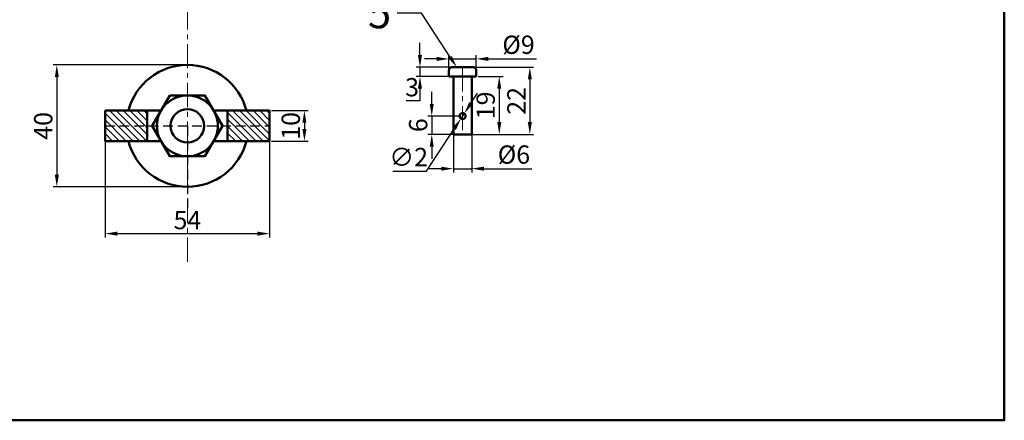
# Model space of a CAD drawing. Units: millimetres. Extents: x -25 to 763, y -62 to 306.
# Tile 5 of 7: x 440 to 763, y -62 to 69. Entities that reach past the tile are written whole.
import ezdxf
from ezdxf import colors
from ezdxf.entities.mleader import LeaderData, LeaderLine
from ezdxf.math import Vec2, Vec3

# ---------------------------------------------------------------- set-up
doc = ezdxf.new("R2010")
doc.units = ezdxf.units.MM
doc.header["$LTSCALE"] = 0.5
doc.linetypes.add('CENTER', pattern=[50.8, 31.75, -6.35, 6.35, -6.35])
doc.linetypes.add('DASHED', pattern=[19.05, 12.7, -6.35])
for name, color, linetype, lineweight in [('M-CNTR', 1, 'CENTER', 18), ('M-DIMS', 2, 'Continuous', 25), ('M-HATC', 8, 'Continuous', 18), ('M-HIDN', 4, 'DASHED', 25), ('M-OUTL', 7, 'Continuous', 50), ('M-TEXT', 3, 'Continuous', 25), ('M-TTLB', 7, 'Continuous', 50)]:
    doc.layers.add(name, color=color, linetype=linetype, lineweight=lineweight)
doc.styles.get("Standard").update_dxf_attribs({"font": 'arial.ttf'})
doc.dimstyles.new('ISO-25', dxfattribs={"dimtxt": 6, "dimasz": 4, "dimexe": 1.25, "dimexo": 0.625, "dimtad": 1, "dimtoh": 1, "dimdec": 1, "dimtxsty": 'Standard', "dimcen": 2.5, "dimadec": 0, "dimazin": 0, "dimtfac": 1, "dimtdec": 1, "dimtmove": 0, "dimatfit": 3, "dimfxl": 1, "dimarcsym": 0})

# ---------------------------------------------------------------- blocks, each defined once
blk = doc.blocks.new('*D17')
at = {"layer": 'Defpoints', "color": 0, "ltscale": 0.5, "transparency": 16777216}
for p in [(468.18, 34.2), (522.18, 34.2), (522.18, -1.17)]:
    blk.add_point(p, dxfattribs=at)
at = {"layer": 'M-DIMS', "color": 0, "lineweight": -2, "ltscale": 0.5, "transparency": 16777216}
for p, q in [((468.18, 33.58), (468.18, -2.42)), ((522.18, 33.58), (522.18, -2.42)), ((472.18, -1.17), (518.18, -1.17))]:
    blk.add_line(p, q, dxfattribs=at)
at = {"layer": 'M-DIMS', "color": 0, "ltscale": 0.5, "transparency": 16777216}
for points in [[(472.18, -0.51), (472.18, -1.84), (468.18, -1.17)], [(518.18, -0.51), (518.18, -1.84), (522.18, -1.17)]]:
    blk.add_solid(points, dxfattribs=at)
at = {"layer": 'M-DIMS', "color": 0, "ltscale": 0.5, "transparency": 16777216, "insert": (495.18, 2.5), "char_height": 6, "attachment_point": 5}
blk.add_mtext('54', dxfattribs=at)
blk = doc.blocks.new('*D18')
at = {"layer": 'Defpoints', "color": 0, "ltscale": 0.5, "transparency": 16777216}
for p in [(495.18, 54.2), (452.33, 14.2), (495.18, 14.2)]:
    blk.add_point(p, dxfattribs=at)
at = {"layer": 'M-DIMS', "color": 0, "lineweight": -2, "ltscale": 0.5, "transparency": 16777216}
for p, q in [((494.55, 54.2), (451.08, 54.2)), ((452.33, 50.2), (452.33, 18.2)), ((494.55, 14.2), (451.08, 14.2))]:
    blk.add_line(p, q, dxfattribs=at)
at = {"layer": 'M-DIMS', "color": 0, "ltscale": 0.5, "transparency": 16777216}
for points in [[(451.66, 50.2), (453, 50.2), (452.33, 54.2)], [(451.66, 18.2), (453, 18.2), (452.33, 14.2)]]:
    blk.add_solid(points, dxfattribs=at)
at = {"layer": 'M-DIMS', "color": 0, "ltscale": 0.5, "transparency": 16777216, "insert": (448.64, 34.2), "char_height": 6, "attachment_point": 5, "rotation": 90}
blk.add_mtext('40', dxfattribs=at)
blk = doc.blocks.new('*D41')
at = {"layer": 'Defpoints', "color": 0, "ltscale": 0.5, "transparency": 16777216}
for p in [(522.18, 39.2), (522.18, 29.2), (533.58, 29.2)]:
    blk.add_point(p, dxfattribs=at)
at = {"layer": 'M-DIMS', "color": 0, "lineweight": -2, "ltscale": 0.5, "transparency": 16777216}
for p, q in [((522.8, 39.2), (534.83, 39.2)), ((533.58, 35.2), (533.58, 33.2)), ((522.8, 29.2), (534.83, 29.2))]:
    blk.add_line(p, q, dxfattribs=at)
at = {"layer": 'M-DIMS', "color": 0, "ltscale": 0.5, "transparency": 16777216}
for points in [[(532.91, 35.2), (534.25, 35.2), (533.58, 39.2)], [(532.91, 33.2), (534.25, 33.2), (533.58, 29.2)]]:
    blk.add_solid(points, dxfattribs=at)
at = {"layer": 'M-DIMS', "color": 0, "ltscale": 0.5, "transparency": 16777216, "insert": (529.89, 34.2), "char_height": 6, "attachment_point": 5, "rotation": 90}
blk.add_mtext('10', dxfattribs=at)
blk = doc.blocks.new('*D55')
at = {"layer": 'Defpoints', "color": 0, "ltscale": 0.5, "transparency": 16777216}
for p in [(589.99, 56.18), (580.99, 51.42), (589.99, 51.42)]:
    blk.add_point(p, dxfattribs=at)
at = {"layer": 'M-DIMS', "color": 0, "lineweight": -2, "ltscale": 0.5, "transparency": 16777216}
for p, q in [((576.99, 56.18), (572.99, 56.18)), ((580.99, 52.04), (580.99, 57.43)), ((580.99, 56.18), (589.99, 56.18)), ((589.99, 52.04), (589.99, 57.43)), ((593.99, 56.18), (609.72, 56.18))]:
    blk.add_line(p, q, dxfattribs=at)
at = {"layer": 'M-DIMS', "color": 0, "ltscale": 0.5, "transparency": 16777216}
for points in [[(576.99, 56.85), (576.99, 55.51), (580.99, 56.18)], [(593.99, 56.85), (593.99, 55.51), (589.99, 56.18)]]:
    blk.add_solid(points, dxfattribs=at)
at = {"layer": 'M-DIMS', "color": 0, "ltscale": 0.5, "transparency": 16777216, "insert": (603.85, 60.04), "char_height": 6, "attachment_point": 5}
blk.add_mtext('%%C9', dxfattribs=at)
blk = doc.blocks.new('*D56')
at = {"layer": 'Defpoints', "color": 0, "ltscale": 0.5, "transparency": 16777216}
for p in [(583.59, 53.42), (571.51, 50.42), (583.59, 50.42)]:
    blk.add_point(p, dxfattribs=at)
at = {"layer": 'M-DIMS', "color": 0, "lineweight": -2, "ltscale": 0.5, "transparency": 16777216}
for p, q in [((571.51, 57.42), (571.51, 61.42)), ((582.97, 53.42), (570.26, 53.42)), ((571.51, 53.42), (571.51, 50.42)), ((582.97, 50.42), (570.26, 50.42)), ((571.51, 46.42), (571.51, 42.42)), ((571.51, 42.42), (566.96, 42.42))]:
    blk.add_line(p, q, dxfattribs=at)
at = {"layer": 'M-DIMS', "color": 0, "ltscale": 0.5, "transparency": 16777216}
for points in [[(570.84, 57.42), (572.18, 57.42), (571.51, 53.42)], [(570.84, 46.42), (572.18, 46.42), (571.51, 50.42)]]:
    blk.add_solid(points, dxfattribs=at)
at = {"layer": 'M-DIMS', "color": 0, "ltscale": 0.5, "transparency": 16777216, "insert": (568.92, 46.11), "char_height": 6, "attachment_point": 5}
blk.add_mtext('3', dxfattribs=at)
blk = doc.blocks.new('*D57')
at = {"layer": 'Defpoints', "color": 0, "ltscale": 0.5, "transparency": 16777216}
for p in [(589.99, 50.42), (588.49, 31.42), (597.54, 31.42)]:
    blk.add_point(p, dxfattribs=at)
at = {"layer": 'M-DIMS', "color": 0, "lineweight": -2, "ltscale": 0.5, "transparency": 16777216}
for p, q in [((590.62, 50.42), (598.79, 50.42)), ((597.54, 46.42), (597.54, 35.42)), ((589.12, 31.42), (598.79, 31.42))]:
    blk.add_line(p, q, dxfattribs=at)
at = {"layer": 'M-DIMS', "color": 0, "ltscale": 0.5, "transparency": 16777216}
for points in [[(596.87, 46.42), (598.2, 46.42), (597.54, 50.42)], [(596.87, 35.42), (598.2, 35.42), (597.54, 31.42)]]:
    blk.add_solid(points, dxfattribs=at)
at = {"layer": 'M-DIMS', "color": 0, "ltscale": 0.5, "transparency": 16777216, "insert": (593.85, 40.92), "char_height": 6, "attachment_point": 5, "rotation": 90}
blk.add_mtext('19', dxfattribs=at)
blk = doc.blocks.new('*D58')
at = {"layer": 'Defpoints', "color": 0, "ltscale": 0.5, "transparency": 16777216}
for p in [(585.49, 53.42), (585.49, 31.42), (607.57, 31.42)]:
    blk.add_point(p, dxfattribs=at)
at = {"layer": 'M-DIMS', "color": 0, "lineweight": -2, "ltscale": 0.5, "transparency": 16777216}
for p, q in [((586.12, 53.42), (608.82, 53.42)), ((607.57, 49.42), (607.57, 35.42)), ((586.12, 31.42), (608.82, 31.42))]:
    blk.add_line(p, q, dxfattribs=at)
at = {"layer": 'M-DIMS', "color": 0, "ltscale": 0.5, "transparency": 16777216}
for points in [[(606.91, 49.42), (608.24, 49.42), (607.57, 53.42)], [(606.91, 35.42), (608.24, 35.42), (607.57, 31.42)]]:
    blk.add_solid(points, dxfattribs=at)
at = {"layer": 'M-DIMS', "color": 0, "ltscale": 0.5, "transparency": 16777216, "insert": (603.94, 42.42), "char_height": 6, "attachment_point": 5, "rotation": 90}
blk.add_mtext('22', dxfattribs=at)
blk = doc.blocks.new('*D59')
at = {"layer": 'Defpoints', "color": 0, "ltscale": 0.5, "transparency": 16777216}
for p in [(585.49, 37.42), (575.38, 31.42), (585.49, 31.42)]:
    blk.add_point(p, dxfattribs=at)
at = {"layer": 'M-DIMS', "color": 0, "lineweight": -2, "ltscale": 0.5, "transparency": 16777216}
for p, q in [((575.38, 41.42), (575.38, 45.42)), ((584.87, 37.42), (574.13, 37.42)), ((575.38, 37.42), (575.38, 31.42)), ((584.87, 31.42), (574.13, 31.42)), ((575.38, 27.42), (575.38, 23.42))]:
    blk.add_line(p, q, dxfattribs=at)
at = {"layer": 'M-DIMS', "color": 0, "ltscale": 0.5, "transparency": 16777216}
for points in [[(574.71, 41.42), (576.04, 41.42), (575.38, 37.42)], [(574.71, 27.42), (576.04, 27.42), (575.38, 31.42)]]:
    blk.add_solid(points, dxfattribs=at)
at = {"layer": 'M-DIMS', "color": 0, "ltscale": 0.5, "transparency": 16777216, "insert": (571.69, 34.42), "char_height": 6, "attachment_point": 5, "rotation": 90}
blk.add_mtext('6', dxfattribs=at)
blk = doc.blocks.new('*D60')
at = {"layer": 'Defpoints', "color": 0, "ltscale": 0.5, "transparency": 16777216}
for p in [(582.49, 44.76), (588.49, 44.76), (588.49, 20.15)]:
    blk.add_point(p, dxfattribs=at)
at = {"layer": 'M-DIMS', "color": 0, "lineweight": -2, "ltscale": 0.5, "transparency": 16777216}
for p, q in [((582.49, 44.14), (582.49, 18.9)), ((588.49, 44.14), (588.49, 18.9)), ((578.49, 20.15), (574.49, 20.15)), ((582.49, 20.15), (588.49, 20.15)), ((592.49, 20.15), (608.2, 20.15))]:
    blk.add_line(p, q, dxfattribs=at)
at = {"layer": 'M-DIMS', "color": 0, "ltscale": 0.5, "transparency": 16777216}
for points in [[(578.49, 20.81), (578.49, 19.48), (582.49, 20.15)], [(592.49, 20.81), (592.49, 19.48), (588.49, 20.15)]]:
    blk.add_solid(points, dxfattribs=at)
at = {"layer": 'M-DIMS', "color": 0, "ltscale": 0.5, "transparency": 16777216, "insert": (602.35, 24), "char_height": 6, "attachment_point": 5}
blk.add_mtext('%%C6', dxfattribs=at)
blk = doc.blocks.new('*D61')
at = {"layer": 'Defpoints', "color": 0, "ltscale": 0.5, "transparency": 16777216}
for p in [(584.94, 36.58), (586.04, 38.26)]:
    blk.add_point(p, dxfattribs=at)
at = {"layer": 'M-DIMS', "color": 0, "lineweight": -2, "ltscale": 0.5, "transparency": 16777216}
for p, q in [((588.24, 41.6), (590.43, 44.94)), ((586.04, 38.26), (584.94, 36.58)), ((573.62, 19.32), (582.75, 33.24)), ((562.59, 19.32), (573.62, 19.32))]:
    blk.add_line(p, q, dxfattribs=at)
at = {"layer": 'M-DIMS', "color": 0, "ltscale": 0.5, "transparency": 16777216}
for points in [[(587.68, 41.97), (588.79, 41.23), (586.04, 38.26)], [(582.19, 33.61), (583.31, 32.87), (584.94, 36.58)]]:
    blk.add_solid(points, dxfattribs=at)
at = {"layer": 'M-DIMS', "color": 0, "ltscale": 0.5, "transparency": 16777216, "insert": (567.79, 23.18), "char_height": 6, "attachment_point": 5}
blk.add_mtext('∅2', dxfattribs=at)

msp = doc.modelspace()

# ---------------------------------------------------------------- hatches: boundary and pattern name
at = {"layer": 'M-HATC', "ltscale": 0.5}
h = msp.add_hatch(dxfattribs=at)
h.set_pattern_fill('ANSI31', color=256, scale=0.5, angle=90)
h.set_pattern_definition([(135, (-56.0338, -32.3511), (-1.122532, -1.122532), [])])
h.paths.add_polyline_path([(489.68, 109.08), (484.68, 109.08, -0.414214), (479.68, 114.08), (479.68, 119.08), (468.68, 119.08), (468.68, 106.08, 0.414214), (473.68, 101.08), (475.68, 101.08, -0.414214), (477.68, 99.08), (481.46, 99.08), (489.68, 99.08)])
h.paths.add_polyline_path([(489.68, 85.08), (481.98, 85.08), (482.98, 85.38), (481.98, 85.96), (482.98, 86.54), (481.98, 87.13), (482.98, 87.7), (481.98, 88.28), (482.98, 88.86), (481.98, 89.43), (482.98, 90.01), (481.98, 90.6), (482.98, 91.18), (481.98, 91.76), (482.98, 92.33), (481.98, 92.91), (482.98, 93.49), (481.98, 94.08), (489.68, 94.08)])
h.paths.add_polyline_path([(489.68, 99.08), (481.46, 99.08), (477.68, 99.08, 1), (477.68, 94.08), (489.68, 94.08)])
h.paths.add_polyline_path([(521.68, 106.08), (521.68, 119.08), (510.68, 119.08), (510.68, 114.08, -0.414214), (505.68, 109.08), (500.68, 109.08), (500.68, 99.08), (512.68, 99.08, -0.414214), (514.68, 101.08), (516.68, 101.08, 0.414214)])
h.paths.add_polyline_path([(512.68, 99.08), (500.68, 99.08), (500.68, 94.08), (512.68, 94.08, 1)])
h.paths.add_polyline_path([(508.38, 94.08), (500.68, 94.08), (500.68, 85.08), (508.38, 85.08), (507.38, 85.38), (508.38, 85.96), (507.38, 86.54), (508.38, 87.13), (507.38, 87.7), (508.38, 88.28), (507.38, 88.86), (508.38, 89.43), (507.38, 90.01), (508.38, 90.6), (507.38, 91.18), (508.38, 91.76), (507.38, 92.33), (508.38, 92.91), (507.38, 93.49)])
h.paths.add_polyline_path([(522.18, 39.2), (508.38, 39.2), (508.38, 34.2), (522.18, 34.2)])
h.paths.add_polyline_path([(522.18, 34.2), (508.38, 34.2), (508.38, 29.2), (522.18, 29.2)])
h.paths.add_polyline_path([(481.98, 39.2), (468.18, 39.2), (468.18, 34.2), (481.98, 34.2)])
h.paths.add_polyline_path([(481.98, 34.2), (468.18, 34.2), (468.18, 29.2), (481.98, 29.2)])

# ---------------------------------------------------------------- linework, layer by layer
at = {"layer": 'M-CNTR', "ltscale": 0.5}
for p, q in [((495.18, -10.41), (495.18, 157.83)), ((585.49, 53.42), (585.49, 31.42))]:
    msp.add_line(p, q, dxfattribs=at)
at = {"layer": 'M-HIDN', "ltscale": 0.5}
for p, q in [((468.18, 34.2), (522.18, 34.2)), ((495.18, 34.2), (495.18, 6.07))]:
    msp.add_line(p, q, dxfattribs=at)
at = {"layer": 'M-OUTL', "ltscale": 0.5}
for p, q in [((580.99, 50.42), (580.99, 52.42)), ((581.99, 53.42), (588.99, 53.42)), ((589.99, 52.42), (589.99, 50.42)), ((589.99, 50.42), (580.99, 50.42)), ((582.49, 31.42), (582.49, 50.42)), ((588.49, 31.42), (588.49, 50.42)), ((468.18, 39.2), (468.18, 29.2)), ((468.18, 39.2), (481.98, 39.2)), ((481.98, 39.2), (481.98, 29.2)), ((481.98, 39.2), (486.52, 39.2)), ((508.38, 39.2), (503.84, 39.2)), ((508.38, 39.2), (522.18, 39.2)), ((508.38, 39.2), (508.38, 29.2)), ((522.18, 39.2), (522.18, 29.2)), ((468.18, 29.2), (481.98, 29.2)), ((481.98, 29.2), (486.52, 29.2)), ((508.38, 29.2), (503.84, 29.2)), ((508.38, 29.2), (522.18, 29.2)), ((582.49, 31.42), (588.49, 31.42))]:
    msp.add_line(p, q, dxfattribs=at)
msp.add_lwpolyline([(489.41, 44.2), (483.63, 34.2), (489.41, 24.2), (500.95, 24.2), (506.73, 34.2), (500.95, 44.2)], close=True, dxfattribs=at)
for centre, radius in [((495.18, 34.2), 10), ((495.18, 34.2), 5.5), ((585.49, 37.42), 1)]:
    msp.add_circle(centre, radius, dxfattribs=at)
for centre, radius, start, end in [((495.18, 34.2), 20, 14.4775, 165.5225), ((581.99, 52.42), 1, 90, 180), ((588.99, 52.42), 1, 0, 90), ((495.18, 34.2), 20, 194.4775, 345.5225)]:
    msp.add_arc(centre, radius, start, end, dxfattribs=at)
at = {"layer": 'M-TTLB', "ltscale": 0.5}
msp.add_lwpolyline([(229.22, 305.74), (763.29, 305.74), (763.29, -62.45), (229.22, -62.45)], close=True, dxfattribs=at)

# ---------------------------------------------------------------- dimensions: what is measured, and where the dimension line sits
at = {"layer": 'M-DIMS', "ltscale": 0.5}
for base, p1, p2, picture, middle in [((571.51, 50.42), (583.59, 53.42), (583.59, 50.42), '*D56', (568.92, 46.11)), ((452.33, 14.2), (495.18, 54.2), (495.18, 14.2), '*D18', (448.64, 34.2)), ((607.57, 31.42), (585.49, 53.42), (585.49, 31.42), '*D58', (603.94, 42.42)), ((597.54, 31.42), (589.99, 50.42), (588.49, 31.42), '*D57', (593.85, 40.92)), ((575.38, 31.42), (585.49, 37.42), (585.49, 31.42), '*D59', (571.69, 34.42)), ((533.58, 29.2), (522.18, 39.2), (522.18, 29.2), '*D41', (529.89, 34.2))]:
    dim = msp.add_linear_dim(base=base, p1=p1, p2=p2, angle=90, dimstyle='ISO-25', override={"dimclrd": 0, "dimclre": 0, "dimclrt": 0}, dxfattribs=at)
    dim.commit()
    dim.dimension.update_dxf_attribs({"geometry": picture, "text_midpoint": middle})
for base, p1, p2, picture, middle in [((589.99, 56.18), (580.99, 51.42), (589.99, 51.42), '*D55', (603.85, 60.04)), ((588.49, 20.15), (582.49, 44.76), (588.49, 44.76), '*D60', (602.35, 24))]:
    dim = msp.add_linear_dim(base=base, p1=p1, p2=p2, text='%%C<>', dimstyle='ISO-25', override={"dimclrd": 0, "dimclre": 0, "dimclrt": 0}, dxfattribs=at)
    dim.commit()
    dim.dimension.update_dxf_attribs({"geometry": picture, "text_midpoint": middle})
dim = msp.add_diameter_dim_2p(p1=(586.04, 38.26), p2=(584.94, 36.58), dimstyle='ISO-25', override={"dimclrd": 0, "dimclre": 0, "dimclrt": 0}, dxfattribs=at)
dim.commit()
dim.dimension.update_dxf_attribs({"geometry": '*D61', "text_midpoint": (567.79, 19.32), "dimtype": 163})
dim = msp.add_linear_dim(base=(522.18, -1.17), p1=(468.18, 34.2), p2=(522.18, 34.2), dimstyle='ISO-25', override={"dimclrd": 0, "dimclre": 0, "dimclrt": 0}, dxfattribs=at)
dim.commit()
dim.dimension.update_dxf_attribs({"geometry": '*D17', "text_midpoint": (495.18, 2.5)})

# ---------------------------------------------------------------- leaders
at = {"layer": 'M-TEXT', "ltscale": 0.5}
ml = msp.add_multileader_mtext('Standard', dxfattribs=at)
ml.set_content('5', color=256)
ml.set_leader_properties()
ml.build(insert=Vec2(0, 0))
ctx = ml.context
ctx.base_point, ctx.char_height, ctx.plane_origin = Vec3(553.41, 71.15), 10, Vec3(583.59, 53.42)
ctx.text_align_type = 2
notes = []
notes.append((ctx, [(0, (1, 1, 0), (572.04, 71.15), (-1, 0), 8, [(0, [(583.59, 53.42)], 0, [])])]))
ctx.mtext.insert, ctx.mtext.alignment, ctx.mtext.flow_direction = Vec3(562.04, 76.23), 3, 5
for ctx, leaders in notes:
    for number, flags, end, landing, length, lines in leaders:
        leader = LeaderData()
        leader.index, (leader.has_last_leader_line, leader.has_dogleg_vector, leader.attachment_direction) = number, flags
        leader.last_leader_point, leader.dogleg_vector, leader.dogleg_length = Vec3(end), Vec3(landing), length
        for number, points, colour, breaks in lines:
            line = LeaderLine()
            line.index, line.vertices, line.color, line.breaks = number, Vec3.list(points), colors.encode_raw_color(colour), breaks
            leader.lines.append(line)
        ctx.leaders.append(leader)

doc.saveas('drawing.dxf')
